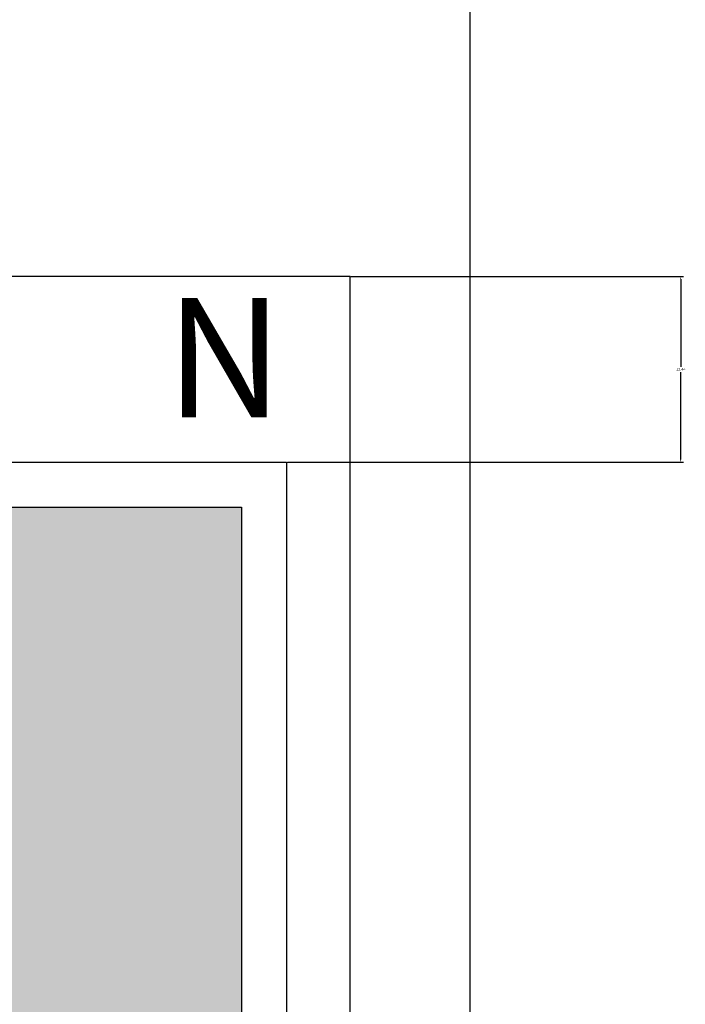
# Model space of a CAD drawing. Units: millimetres. Extents: x -8 to 285, y 5 to 221.
# Tile 22 of 30: x 241 to 285, y 66 to 132. Entities that reach past the tile are written whole.
import ezdxf

# ---------------------------------------------------------------- set-up
doc = ezdxf.new("R2010")
doc.units = ezdxf.units.MM
for name, color, linetype, lineweight in [('A-ANNO-DIMS', 2, 'Continuous', 18), ('E-ANNO-TEXT', 7, 'Continuous', 18), ('E-EQPM-PATT', 252, 'Continuous', 13), ('E-POWR-AC-NEUT', 3, 'Continuous', 25), ('E-POWR-INVR', 7, 'Continuous', 30)]:
    doc.layers.add(name, color=color, linetype=linetype, lineweight=lineweight)
doc.layers.add('E-POWR-AC-LINE', color=30, linetype='Continuous', lineweight=25, true_color=0xf26722)
doc.styles.get("Standard").update_dxf_attribs({"font": 'arial.ttf'})
doc.dimstyles.get("Standard").update_dxf_attribs({"dimtxt": 0.18, "dimasz": 0.18, "dimexe": 0.18, "dimexo": 0.0625, "dimgap": 0.09, "dimtad": 0, "dimtih": 1, "dimtoh": 1, "dimdec": 4, "dimzin": 0, "dimdsep": 46, "dimtxsty": 'Standard', "dimcen": 0.09, "dimadec": 0, "dimazin": 0, "dimtfac": 1, "dimtdec": 4, "dimtofl": 0, "dimtmove": 0, "dimatfit": 3, "dimfxl": 1, "dimtolj": 1, "dimtzin": 0, "dimarcsym": 0})

# ---------------------------------------------------------------- blocks, each defined once
blk = doc.blocks.new('*D28')
at = {"layer": 'A-ANNO-DIMS', "color": 0, "lineweight": -2, "transparency": 16777216}
for p, q in [((262.935, 115.143), (285.199, 115.143)), ((285.019, 114.963), (285.019, 109.103)), ((285.019, 102.882), (285.019, 108.742)), ((258.678, 102.702), (285.199, 102.702))]:
    blk.add_line(p, q, dxfattribs=at)
at = {"layer": 'A-ANNO-DIMS', "color": 0, "transparency": 16777216}
for points in [[(284.989, 114.963), (285.049, 114.963), (285.019, 115.143)], [(284.989, 102.882), (285.049, 102.882), (285.019, 102.702)]]:
    blk.add_solid(points, dxfattribs=at)
at = {"layer": 'Defpoints', "color": 0, "transparency": 16777216}
for p in [(262.873, 115.143), (285.019, 115.143), (258.615, 102.702)]:
    blk.add_point(p, dxfattribs=at)
at = {"layer": 'A-ANNO-DIMS', "color": 0, "transparency": 16777216, "insert": (285.019, 108.922), "char_height": 0.18, "attachment_point": 5}
blk.add_mtext('\\A1;12.44', dxfattribs=at)

msp = doc.modelspace()

# ---------------------------------------------------------------- hatches: boundary and pattern name
at = {"layer": 'E-EQPM-PATT'}
h = msp.add_hatch(color=256, dxfattribs=at)
h.set_gradient(color1=(175, 217, 170), color2=(175, 217, 170), tint=1)
h.paths.add_polyline_path([(255.6152, 99.7021), (190.9955, 99.7021), (190.9955, 53.4644), (215.8749, 53.4644), (215.8749, 47.6512), (217.2608, 47.6512), (219.2608, 45.6512), (219.2608, 32.6512), (199.2608, 32.6512), (199.2608, 44.4759), (190.9955, 44.4759), (190.9955, 28.2311), (237.8513, 28.2311), (237.8513, 32.6512), (231.5468, 32.6512, -0.5773503), (229.8147, 35.6512), (231.5468, 38.6512), (231.5468, 58.5666), (255.6152, 58.5666)])
h.paths.add_polyline_path([(208.2775, 92.6953), (238.0827, 92.6953), (238.0827, 67.6708), (208.2775, 67.6708)], flags=16)
h.paths.add_polyline_path([(213.1801, 80.183, -1), (233.1801, 80.183, -1)], flags=0)
h.paths.add_polyline_path([(215.1801, 80.183, -1), (231.1801, 80.183, -1)], flags=0)
h.paths.add_polyline_path([(217.1801, 80.183, -1), (229.1801, 80.183, -1)], flags=0)
h.paths.add_polyline_path([(219.1801, 80.183, -1), (227.1801, 80.183, -1)], flags=0)
h.paths.add_polyline_path([(255.6152, 58.5666), (231.5468, 58.5666), (231.5468, 38.6512), (236.3506, 46.9717, -0.5773503), (239.8147, 46.9717), (244.6186, 38.6512), (244.6186, 49.925), (255.6152, 49.925)], flags=17)
h.paths.add_polyline_path([(215.8749, 53.4644), (190.9955, 53.4644), (190.9955, 48.962), (202.4345, 48.962), (202.4345, 47.6512), (215.8749, 47.6512)], flags=17)
h.paths.add_polyline_path([(255.6152, 49.925), (244.6186, 49.925), (244.6186, 38.6512), (246.3506, 35.6512, -0.5773503), (244.6186, 32.6512), (237.8513, 32.6512), (237.8513, 28.2311), (190.9955, 28.2311), (190.9955, 25.6297), (255.6152, 25.6297)])
h.paths.add_polyline_path([(199.2608, 45.6512), (201.2608, 47.6512), (202.4345, 47.6512), (202.4345, 48.962), (190.9955, 48.962), (190.9955, 44.4759), (199.2608, 44.4759)], flags=17)

# ---------------------------------------------------------------- linework, layer by layer
at = {"layer": 'E-POWR-AC-LINE'}
msp.add_lwpolyline([(244.6186, 34.6512), (244.6186, 49.925), (270.9192, 49.925), (270.9192, 206.4568), (145.1651, 206.4568), (145.1651, 201.7939)], dxfattribs=at)
at = {"layer": 'E-POWR-AC-NEUT'}
msp.add_lwpolyline([(231.5468, 34.6512), (231.5468, 58.5666), (262.873, 58.5666), (262.873, 115.1427), (144.6762, 115.1427), (144.6762, 130.9614)], dxfattribs=at)
at = {"layer": 'E-POWR-INVR'}
for points in [[(187.9955, 102.7021), (258.6152, 102.7021), (258.6152, 22.6297), (187.9955, 22.6297)], [(190.9955, 99.7021), (255.6152, 99.7021), (255.6152, 25.6297), (190.9955, 25.6297)]]:
    msp.add_lwpolyline(points, close=True, dxfattribs=at)

# ---------------------------------------------------------------- texts
at = {"layer": 'E-ANNO-TEXT', "insert": (250.5126, 113.7103), "char_height": 8, "attachment_point": 1}
msp.add_mtext_dynamic_manual_height_columns('N', width=11.038304, gutter_width=12.5, heights=[0], dxfattribs=at)

# ---------------------------------------------------------------- dimensions: what is measured, and where the dimension line sits
at = {"layer": 'A-ANNO-DIMS'}
dim = msp.add_linear_dim(base=(285.0192, 115.1427), p1=(258.6152, 102.7021), p2=(262.873, 115.1427), angle=90, dimstyle='Standard', override={"dimdec": 2, "dimlfac": 1, "dimrnd": 0, "dimzin": 0, "dimdsep": 46, "dimlunit": 2}, dxfattribs=at)
dim.commit()
dim.dimension.update_dxf_attribs({"geometry": '*D28', "text_midpoint": (285.0192, 108.9224)})

doc.saveas('drawing.dxf')
